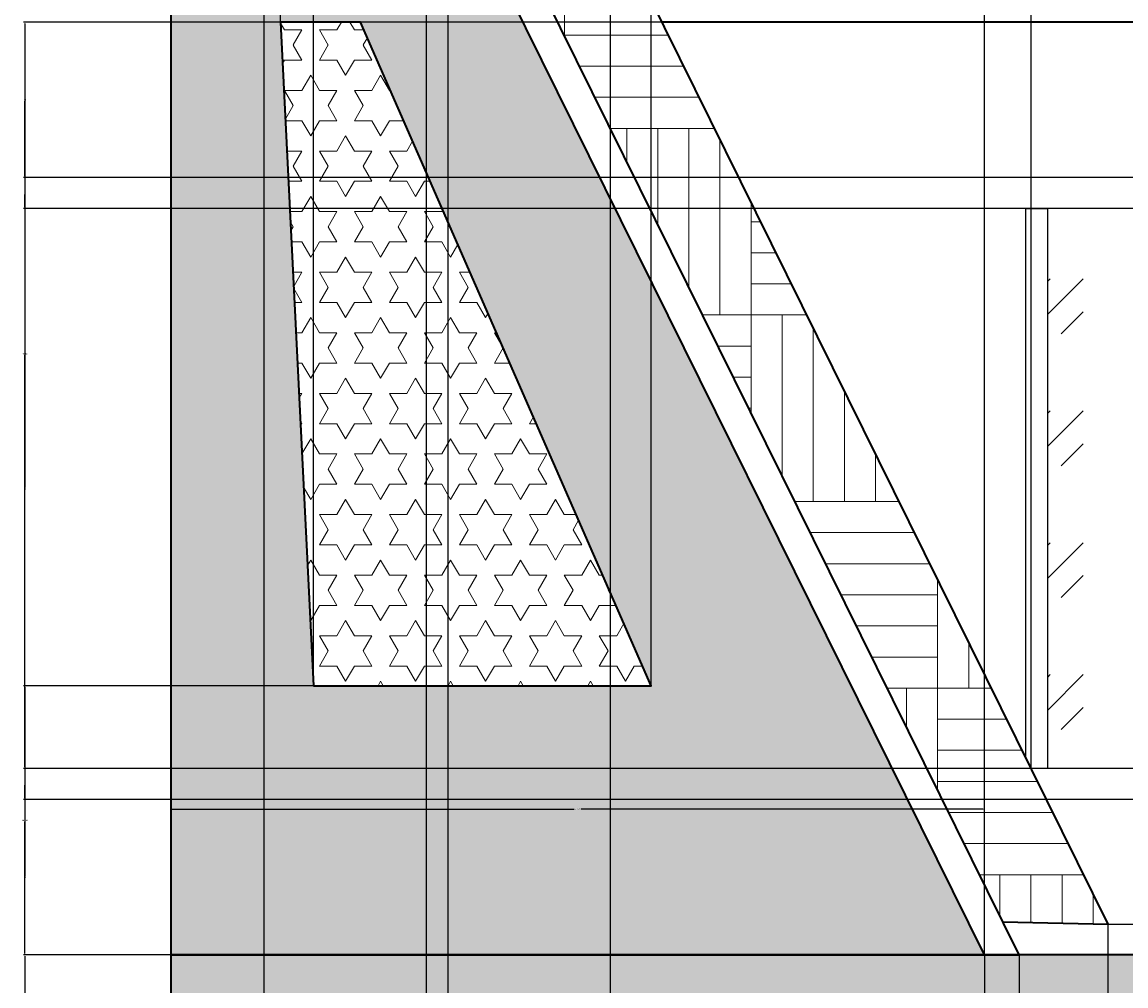
# Model space of a CAD drawing. Units: inches. Extents: x -9 to 389, y -55 to 344.
# Tile 2 of 5: x -9 to 133, y 119 to 243. Entities that reach past the tile are written whole.
import ezdxf

# ---------------------------------------------------------------- set-up
doc = ezdxf.new("R2010")
doc.units = ezdxf.units.IN
doc.header["$MEASUREMENT"] = 0
for name, color, linetype, lineweight in [('A-ANNO-DIMS', 2, 'Continuous', 18), ('A-ELEV', 7, 'Continuous', 35), ('A-ELEV-PATT', 8, 'Continuous', 13), ('A-GLAZ', 4, 'Continuous', 25), ('A-GLAZ-PATT', 252, 'Continuous', 13), ('A-ROOF', 1, 'Continuous', 35), ('A-ROOF-PATT', 8, 'Continuous', 13)]:
    doc.layers.add(name, color=color, linetype=linetype, lineweight=lineweight)
doc.styles.get("Standard").update_dxf_attribs({"font": 'arial.ttf'})
doc.dimstyles.get("Standard").update_dxf_attribs({"dimtxt": 0.18, "dimasz": 0.18, "dimexe": 0.18, "dimexo": 0.0625, "dimgap": 0.09, "dimtad": 0, "dimtih": 1, "dimtoh": 1, "dimdec": 4, "dimzin": 0, "dimdsep": 46, "dimtxsty": 'Standard', "dimcen": 0.09, "dimadec": 0, "dimazin": 0, "dimtfac": 1, "dimtdec": 4, "dimtofl": 0, "dimtmove": 0, "dimatfit": 3, "dimfxl": 1, "dimtolj": 1, "dimtzin": 0, "dimarcsym": 0})

# ---------------------------------------------------------------- blocks, each defined once
blk = doc.blocks.new('*D2')
at = {"layer": 'A-ANNO-DIMS', "color": 0, "lineweight": -2, "transparency": 16777216}
for p, q in [((23.77, 242.83), (23.77, 343.8)), ((23.95, 343.62), (25.5, 343.62)), ((27.83, 343.62), (26.29, 343.62)), ((28.01, 157.47), (28.01, 343.8))]:
    blk.add_line(p, q, dxfattribs=at)
at = {"layer": 'A-ANNO-DIMS', "color": 0, "transparency": 16777216}
for points in [[(23.95, 343.65), (23.95, 343.59), (23.77, 343.62)], [(27.83, 343.65), (27.83, 343.59), (28.01, 343.62)]]:
    blk.add_solid(points, dxfattribs=at)
at = {"layer": 'Defpoints', "color": 0, "transparency": 16777216}
for p in [(28.01, 343.62), (23.77, 242.77), (28.01, 157.4)]:
    blk.add_point(p, dxfattribs=at)
at = {"layer": 'A-ANNO-DIMS', "color": 0, "transparency": 16777216, "insert": (25.89, 343.62), "char_height": 0.18, "attachment_point": 5}
blk.add_mtext('\\A1;4.244', dxfattribs=at)
blk = doc.blocks.new('*D3')
at = {"layer": 'A-ANNO-DIMS', "color": 0, "lineweight": -2, "transparency": 16777216}
for p, q in [((28.01, 157.47), (28.01, 343.8)), ((28.19, 343.62), (49.26, 343.62)), ((71.27, 343.62), (50.2, 343.62)), ((71.45, 157.47), (71.45, 343.8))]:
    blk.add_line(p, q, dxfattribs=at)
at = {"layer": 'A-ANNO-DIMS', "color": 0, "transparency": 16777216}
for points in [[(28.19, 343.65), (28.19, 343.59), (28.01, 343.62)], [(71.27, 343.65), (71.27, 343.59), (71.45, 343.62)]]:
    blk.add_solid(points, dxfattribs=at)
at = {"layer": 'Defpoints', "color": 0, "transparency": 16777216}
for p in [(71.45, 343.62), (28.01, 157.4), (71.45, 157.4)]:
    blk.add_point(p, dxfattribs=at)
at = {"layer": 'A-ANNO-DIMS', "color": 0, "transparency": 16777216, "insert": (49.73, 343.62), "char_height": 0.18, "attachment_point": 5}
blk.add_mtext('\\A1;43.435', dxfattribs=at)
blk = doc.blocks.new('*D4')
at = {"layer": 'A-ANNO-DIMS', "color": 0, "lineweight": -2, "transparency": 16777216}
for p, q in [((71.45, 157.47), (71.45, 343.8)), ((71.63, 343.62), (119.03, 343.62)), ((167.08, 343.62), (119.68, 343.62)), ((167.26, 324.93), (167.26, 343.8))]:
    blk.add_line(p, q, dxfattribs=at)
at = {"layer": 'A-ANNO-DIMS', "color": 0, "transparency": 16777216}
for points in [[(71.63, 343.65), (71.63, 343.59), (71.45, 343.62)], [(167.08, 343.65), (167.08, 343.59), (167.26, 343.62)]]:
    blk.add_solid(points, dxfattribs=at)
at = {"layer": 'Defpoints', "color": 0, "transparency": 16777216}
for p in [(167.26, 343.62), (167.26, 324.87), (71.45, 157.4)]:
    blk.add_point(p, dxfattribs=at)
at = {"layer": 'A-ANNO-DIMS', "color": 0, "transparency": 16777216, "insert": (119.35, 343.62), "char_height": 0.18, "attachment_point": 5}
blk.add_mtext('\\A1;95.8', dxfattribs=at)
blk = doc.blocks.new('*D16')
at = {"layer": 'A-ANNO-DIMS', "color": 0, "lineweight": -2, "transparency": 16777216}
for p, q in [((21.65, 14.83), (21.65, 343.8)), ((21.83, 343.62), (31.64, 343.62)), ((42.37, 343.62), (32.57, 343.62)), ((42.55, 14.83), (42.55, 343.8))]:
    blk.add_line(p, q, dxfattribs=at)
at = {"layer": 'A-ANNO-DIMS', "color": 0, "transparency": 16777216}
for points in [[(21.83, 343.65), (21.83, 343.59), (21.65, 343.62)], [(42.37, 343.65), (42.37, 343.59), (42.55, 343.62)]]:
    blk.add_solid(points, dxfattribs=at)
at = {"layer": 'Defpoints', "color": 0, "transparency": 16777216}
for p in [(42.55, 343.62), (21.65, 14.77), (42.55, 14.77)]:
    blk.add_point(p, dxfattribs=at)
at = {"layer": 'A-ANNO-DIMS', "color": 0, "transparency": 16777216, "insert": (32.1, 343.62), "char_height": 0.18, "attachment_point": 5}
blk.add_mtext('\\A1;20.896', dxfattribs=at)
blk = doc.blocks.new('*D17')
at = {"layer": 'A-ANNO-DIMS', "color": 0, "lineweight": -2, "transparency": 16777216}
for p, q in [((42.55, 14.83), (42.55, 343.8)), ((42.73, 343.62), (43.61, 343.62)), ((45.14, 343.62), (44.26, 343.62)), ((45.32, 14.83), (45.32, 343.8))]:
    blk.add_line(p, q, dxfattribs=at)
at = {"layer": 'A-ANNO-DIMS', "color": 0, "transparency": 16777216}
for points in [[(42.73, 343.65), (42.73, 343.59), (42.55, 343.62)], [(45.14, 343.65), (45.14, 343.59), (45.32, 343.62)]]:
    blk.add_solid(points, dxfattribs=at)
at = {"layer": 'Defpoints', "color": 0, "transparency": 16777216}
for p in [(45.32, 343.62), (42.55, 14.77), (45.32, 14.77)]:
    blk.add_point(p, dxfattribs=at)
at = {"layer": 'A-ANNO-DIMS', "color": 0, "transparency": 16777216, "insert": (43.93, 343.62), "char_height": 0.18, "attachment_point": 5}
blk.add_mtext('\\A1;2.77', dxfattribs=at)
blk = doc.blocks.new('*D18')
at = {"layer": 'A-ANNO-DIMS', "color": 0, "lineweight": -2, "transparency": 16777216}
for p, q in [((45.32, 14.83), (45.32, 343.8)), ((45.5, 343.62), (55.3, 343.62)), ((66.03, 343.62), (56.23, 343.62)), ((66.21, 14.83), (66.21, 343.8))]:
    blk.add_line(p, q, dxfattribs=at)
at = {"layer": 'A-ANNO-DIMS', "color": 0, "transparency": 16777216}
for points in [[(45.5, 343.65), (45.5, 343.59), (45.32, 343.62)], [(66.03, 343.65), (66.03, 343.59), (66.21, 343.62)]]:
    blk.add_solid(points, dxfattribs=at)
at = {"layer": 'Defpoints', "color": 0, "transparency": 16777216}
for p in [(66.21, 343.62), (45.32, 14.77), (66.21, 14.77)]:
    blk.add_point(p, dxfattribs=at)
at = {"layer": 'A-ANNO-DIMS', "color": 0, "transparency": 16777216, "insert": (55.77, 343.62), "char_height": 0.18, "attachment_point": 5}
blk.add_mtext('\\A1;20.896', dxfattribs=at)
blk = doc.blocks.new('*D19')
at = {"layer": 'A-ANNO-DIMS', "color": 0, "lineweight": -2, "transparency": 16777216}
for p, q in [((66.21, 14.83), (66.21, 343.8)), ((66.39, 343.62), (109.71, 343.62)), ((153.81, 343.62), (110.5, 343.62)), ((153.99, 14.83), (153.99, 343.8))]:
    blk.add_line(p, q, dxfattribs=at)
at = {"layer": 'A-ANNO-DIMS', "color": 0, "transparency": 16777216}
for points in [[(66.39, 343.65), (66.39, 343.59), (66.21, 343.62)], [(153.81, 343.65), (153.81, 343.59), (153.99, 343.62)]]:
    blk.add_solid(points, dxfattribs=at)
at = {"layer": 'Defpoints', "color": 0, "transparency": 16777216}
for p in [(153.99, 343.62), (66.21, 14.77), (153.99, 14.77)]:
    blk.add_point(p, dxfattribs=at)
at = {"layer": 'A-ANNO-DIMS', "color": 0, "transparency": 16777216, "insert": (110.1, 343.62), "char_height": 0.18, "attachment_point": 5}
blk.add_mtext('\\A1;87.77', dxfattribs=at)
blk = doc.blocks.new('*D23')
at = {"layer": 'A-ANNO-DIMS', "color": 0, "lineweight": -2, "transparency": 16777216}
for p, q in [((9.59, 122.77), (-9.28, 122.77)), ((-9.1, 122.59), (-9.1, 116.95)), ((-9.1, 110.95), (-9.1, 116.59)), ((21.59, 110.77), (-9.28, 110.77))]:
    blk.add_line(p, q, dxfattribs=at)
at = {"layer": 'A-ANNO-DIMS', "color": 0, "transparency": 16777216}
for points in [[(-9.13, 122.59), (-9.07, 122.59), (-9.1, 122.77)], [(-9.13, 110.95), (-9.07, 110.95), (-9.1, 110.77)]]:
    blk.add_solid(points, dxfattribs=at)
at = {"layer": 'Defpoints', "color": 0, "transparency": 16777216}
for p in [(-9.1, 122.77), (9.65, 122.77), (21.65, 110.77)]:
    blk.add_point(p, dxfattribs=at)
at = {"layer": 'A-ANNO-DIMS', "color": 0, "transparency": 16777216, "insert": (-9.1, 116.77), "char_height": 0.18, "attachment_point": 5}
blk.add_mtext('\\A1;12', dxfattribs=at)
blk = doc.blocks.new('*D24')
at = {"layer": 'A-ANNO-DIMS', "color": 0, "lineweight": -2, "transparency": 16777216}
for p, q in [((27.95, 157.4), (-9.28, 157.4)), ((-9.1, 157.22), (-9.1, 140.27)), ((-9.1, 122.95), (-9.1, 139.9)), ((9.59, 122.77), (-9.28, 122.77))]:
    blk.add_line(p, q, dxfattribs=at)
at = {"layer": 'A-ANNO-DIMS', "color": 0, "transparency": 16777216}
for points in [[(-9.13, 157.22), (-9.07, 157.22), (-9.1, 157.4)], [(-9.13, 122.95), (-9.07, 122.95), (-9.1, 122.77)]]:
    blk.add_solid(points, dxfattribs=at)
at = {"layer": 'Defpoints', "color": 0, "transparency": 16777216}
for p in [(-9.1, 157.4), (28.01, 157.4), (9.65, 122.77)]:
    blk.add_point(p, dxfattribs=at)
at = {"layer": 'A-ANNO-DIMS', "color": 0, "transparency": 16777216, "insert": (-9.1, 140.09), "char_height": 0.18, "attachment_point": 5}
blk.add_mtext('\\A1;34.636', dxfattribs=at)
blk = doc.blocks.new('*D25')
at = {"layer": 'A-ANNO-DIMS', "color": 0, "lineweight": -2, "transparency": 16777216}
for p, q in [((23.71, 242.77), (-9.28, 242.77)), ((-9.1, 242.59), (-9.1, 200.27)), ((-9.1, 157.58), (-9.1, 199.9)), ((27.95, 157.4), (-9.28, 157.4))]:
    blk.add_line(p, q, dxfattribs=at)
at = {"layer": 'A-ANNO-DIMS', "color": 0, "transparency": 16777216}
for points in [[(-9.13, 242.59), (-9.07, 242.59), (-9.1, 242.77)], [(-9.13, 157.58), (-9.07, 157.58), (-9.1, 157.4)]]:
    blk.add_solid(points, dxfattribs=at)
at = {"layer": 'Defpoints', "color": 0, "transparency": 16777216}
for p in [(-9.1, 242.77), (23.77, 242.77), (28.01, 157.4)]:
    blk.add_point(p, dxfattribs=at)
at = {"layer": 'A-ANNO-DIMS', "color": 0, "transparency": 16777216, "insert": (-9.1, 200.09), "char_height": 0.18, "attachment_point": 5}
blk.add_mtext('\\A1;85.36', dxfattribs=at)
blk = doc.blocks.new('*D32')
at = {"layer": 'A-ANNO-DIMS', "color": 0, "lineweight": -2, "transparency": 16777216}
for p, q in [((9.65, 122.83), (9.65, 141.7)), ((9.83, 141.52), (61.53, 141.52)), ((114.14, 141.52), (62.44, 141.52)), ((114.32, 122.83), (114.32, 141.7))]:
    blk.add_line(p, q, dxfattribs=at)
at = {"layer": 'A-ANNO-DIMS', "color": 0, "transparency": 16777216}
for points in [[(9.83, 141.55), (9.83, 141.49), (9.65, 141.52)], [(114.14, 141.55), (114.14, 141.49), (114.32, 141.52)]]:
    blk.add_solid(points, dxfattribs=at)
at = {"layer": 'Defpoints', "color": 0, "transparency": 16777216}
for p in [(114.32, 141.52), (9.65, 122.77), (114.32, 122.77)]:
    blk.add_point(p, dxfattribs=at)
at = {"layer": 'A-ANNO-DIMS', "color": 0, "transparency": 16777216, "insert": (61.99, 141.52), "char_height": 0.18, "attachment_point": 5}
blk.add_mtext('\\A1;104.67', dxfattribs=at)
blk = doc.blocks.new('*D45')
at = {"layer": 'A-ANNO-DIMS', "color": 0, "lineweight": -2, "transparency": 16777216}
for p, q in [((122.22, 142.77), (-9.28, 142.77)), ((-9.1, 142.59), (-9.1, 132.95)), ((-9.1, 122.95), (-9.1, 132.59)), ((114.26, 122.77), (-9.28, 122.77))]:
    blk.add_line(p, q, dxfattribs=at)
at = {"layer": 'A-ANNO-DIMS', "color": 0, "transparency": 16777216}
for points in [[(-9.13, 142.59), (-9.07, 142.59), (-9.1, 142.77)], [(-9.13, 122.95), (-9.07, 122.95), (-9.1, 122.77)]]:
    blk.add_solid(points, dxfattribs=at)
at = {"layer": 'Defpoints', "color": 0, "transparency": 16777216}
for p in [(-9.1, 142.77), (122.28, 142.77), (114.32, 122.77)]:
    blk.add_point(p, dxfattribs=at)
at = {"layer": 'A-ANNO-DIMS', "color": 0, "transparency": 16777216, "insert": (-9.1, 132.77), "char_height": 0.18, "attachment_point": 5}
blk.add_mtext('\\A1;20', dxfattribs=at)
blk = doc.blocks.new('*D46')
at = {"layer": 'A-ANNO-DIMS', "color": 0, "lineweight": -2, "transparency": 16777216}
for p, q in [((120.238568, 146.768105), (-9.276734, 146.768105)), ((-9.096734, 146.588105), (-9.096734, 144.948105)), ((-9.096734, 142.948105), (-9.096734, 144.588105)), ((122.216644, 142.768105), (-9.276734, 142.768105))]:
    blk.add_line(p, q, dxfattribs=at)
at = {"layer": 'A-ANNO-DIMS', "color": 0, "transparency": 16777216}
for points in [[(-9.126734, 146.588105), (-9.066734, 146.588105), (-9.096734, 146.768105)], [(-9.126734, 142.948105), (-9.066734, 142.948105), (-9.096734, 142.768105)]]:
    blk.add_solid(points, dxfattribs=at)
at = {"layer": 'Defpoints', "color": 0, "transparency": 16777216}
for p in [(-9.096734, 146.768105), (120.301068, 146.768105), (122.279144, 142.768105)]:
    blk.add_point(p, dxfattribs=at)
at = {"layer": 'A-ANNO-DIMS', "color": 0, "transparency": 16777216, "insert": (-9.096734, 144.768105), "char_height": 0.18, "attachment_point": 5}
blk.add_mtext('\\A1;4', dxfattribs=at)
blk = doc.blocks.new('*D47')
at = {"layer": 'A-ANNO-DIMS', "color": 0, "lineweight": -2, "transparency": 16777216}
for p, q in [((84.63, 218.77), (-9.28, 218.77)), ((-9.1, 218.59), (-9.1, 182.95)), ((-9.1, 146.95), (-9.1, 182.59)), ((120.24, 146.77), (-9.28, 146.77))]:
    blk.add_line(p, q, dxfattribs=at)
at = {"layer": 'A-ANNO-DIMS', "color": 0, "transparency": 16777216}
for points in [[(-9.13, 218.59), (-9.07, 218.59), (-9.1, 218.77)], [(-9.13, 146.95), (-9.07, 146.95), (-9.1, 146.77)]]:
    blk.add_solid(points, dxfattribs=at)
at = {"layer": 'Defpoints', "color": 0, "transparency": 16777216}
for p in [(-9.1, 218.77), (84.7, 218.77), (120.3, 146.77)]:
    blk.add_point(p, dxfattribs=at)
at = {"layer": 'A-ANNO-DIMS', "color": 0, "transparency": 16777216, "insert": (-9.1, 182.77), "char_height": 0.18, "attachment_point": 5}
blk.add_mtext('\\A1;72', dxfattribs=at)
blk = doc.blocks.new('*D48')
at = {"layer": 'A-ANNO-DIMS', "color": 0, "lineweight": -2, "transparency": 16777216}
for p, q in [((82.655126, 222.768105), (-9.276734, 222.768105)), ((-9.096734, 222.588105), (-9.096734, 220.948105)), ((-9.096734, 218.948105), (-9.096734, 220.588105)), ((84.633202, 218.768105), (-9.276734, 218.768105))]:
    blk.add_line(p, q, dxfattribs=at)
at = {"layer": 'A-ANNO-DIMS', "color": 0, "transparency": 16777216}
for points in [[(-9.126734, 222.588105), (-9.066734, 222.588105), (-9.096734, 222.768105)], [(-9.126734, 218.948105), (-9.066734, 218.948105), (-9.096734, 218.768105)]]:
    blk.add_solid(points, dxfattribs=at)
at = {"layer": 'Defpoints', "color": 0, "transparency": 16777216}
for p in [(-9.096734, 222.768105), (82.717626, 222.768105), (84.695702, 218.768105)]:
    blk.add_point(p, dxfattribs=at)
at = {"layer": 'A-ANNO-DIMS', "color": 0, "transparency": 16777216, "insert": (-9.096734, 220.768105), "char_height": 0.18, "attachment_point": 5}
blk.add_mtext('\\A1;4', dxfattribs=at)
blk = doc.blocks.new('*D49')
at = {"layer": 'A-ANNO-DIMS', "color": 0, "lineweight": -2, "transparency": 16777216}
for p, q in [((72.76, 242.77), (-9.28, 242.77)), ((-9.1, 242.59), (-9.1, 232.95)), ((-9.1, 222.95), (-9.1, 232.59)), ((82.66, 222.77), (-9.28, 222.77))]:
    blk.add_line(p, q, dxfattribs=at)
at = {"layer": 'A-ANNO-DIMS', "color": 0, "transparency": 16777216}
for points in [[(-9.13, 242.59), (-9.07, 242.59), (-9.1, 242.77)], [(-9.13, 222.95), (-9.07, 222.95), (-9.1, 222.77)]]:
    blk.add_solid(points, dxfattribs=at)
at = {"layer": 'Defpoints', "color": 0, "transparency": 16777216}
for p in [(-9.1, 242.77), (72.83, 242.77), (82.72, 222.77)]:
    blk.add_point(p, dxfattribs=at)
at = {"layer": 'A-ANNO-DIMS', "color": 0, "transparency": 16777216, "insert": (-9.1, 232.77), "char_height": 0.18, "attachment_point": 5}
blk.add_mtext('\\A1;20', dxfattribs=at)
blk = doc.blocks.new('*D57')
at = {"layer": 'A-ANNO-DIMS', "color": 0, "lineweight": -2, "transparency": 16777216}
for p, q in [((114.32, 122.83), (114.32, 343.8)), ((114.5, 343.62), (116.93, 343.62)), ((120.12, 343.62), (117.69, 343.62)), ((120.3, 146.83), (120.3, 343.8))]:
    blk.add_line(p, q, dxfattribs=at)
at = {"layer": 'A-ANNO-DIMS', "color": 0, "transparency": 16777216}
for points in [[(114.5, 343.65), (114.5, 343.59), (114.32, 343.62)], [(120.12, 343.65), (120.12, 343.59), (120.3, 343.62)]]:
    blk.add_solid(points, dxfattribs=at)
at = {"layer": 'Defpoints', "color": 0, "transparency": 16777216}
for p in [(120.3, 343.62), (120.3, 146.77), (114.32, 122.77)]:
    blk.add_point(p, dxfattribs=at)
at = {"layer": 'A-ANNO-DIMS', "color": 0, "transparency": 16777216, "insert": (117.31, 343.62), "char_height": 0.18, "attachment_point": 5}
blk.add_mtext('\\A1;5.981', dxfattribs=at)
blk = doc.blocks.new('*D58')
at = {"layer": 'A-ANNO-DIMS', "color": 0, "lineweight": -2, "transparency": 16777216}
for p, q in [((120.3, 146.83), (120.3, 343.8)), ((120.48, 343.62), (131.33, 343.62)), ((143.12, 343.62), (132.26, 343.62)), ((143.3, 146.83), (143.3, 343.8))]:
    blk.add_line(p, q, dxfattribs=at)
at = {"layer": 'A-ANNO-DIMS', "color": 0, "transparency": 16777216}
for points in [[(120.48, 343.65), (120.48, 343.59), (120.3, 343.62)], [(143.12, 343.65), (143.12, 343.59), (143.3, 343.62)]]:
    blk.add_solid(points, dxfattribs=at)
at = {"layer": 'Defpoints', "color": 0, "transparency": 16777216}
for p in [(143.3, 343.62), (120.3, 146.77), (143.3, 146.77)]:
    blk.add_point(p, dxfattribs=at)
at = {"layer": 'A-ANNO-DIMS', "color": 0, "transparency": 16777216, "insert": (131.8, 343.62), "char_height": 0.18, "attachment_point": 5}
blk.add_mtext('\\A1;22.994', dxfattribs=at)
blk = doc.blocks.new('*D64')
at = {"layer": 'A-ANNO-DIMS', "color": 0, "lineweight": -2, "transparency": 16777216}
for p, q in [((130.27, 126.74), (388.58, 126.74)), ((388.4, 126.56), (388.4, 124.94)), ((388.4, 122.95), (388.4, 124.57)), ((118.84, 122.77), (388.58, 122.77))]:
    blk.add_line(p, q, dxfattribs=at)
at = {"layer": 'A-ANNO-DIMS', "color": 0, "transparency": 16777216}
for points in [[(388.37, 126.56), (388.43, 126.56), (388.4, 126.74)], [(388.37, 122.95), (388.43, 122.95), (388.4, 122.77)]]:
    blk.add_solid(points, dxfattribs=at)
at = {"layer": 'Defpoints', "color": 0, "transparency": 16777216}
for p in [(130.2, 126.74), (388.4, 126.74), (118.78, 122.77)]:
    blk.add_point(p, dxfattribs=at)
at = {"layer": 'A-ANNO-DIMS', "color": 0, "transparency": 16777216, "insert": (388.4, 124.76), "char_height": 0.18, "attachment_point": 5}
blk.add_mtext('\\A1;3.976', dxfattribs=at)
blk = doc.blocks.new('*D65')
at = {"layer": 'A-ANNO-DIMS', "color": 0, "lineweight": -2, "transparency": 16777216}
for p, q in [((130.2, 126.68), (130.2, -54.92)), ((118.78, 122.71), (118.78, -54.92)), ((118.96, -54.74), (124.11, -54.74)), ((130.02, -54.74), (124.88, -54.74))]:
    blk.add_line(p, q, dxfattribs=at)
at = {"layer": 'A-ANNO-DIMS', "color": 0, "transparency": 16777216}
for points in [[(118.96, -54.71), (118.96, -54.77), (118.78, -54.74)], [(130.02, -54.71), (130.02, -54.77), (130.2, -54.74)]]:
    blk.add_solid(points, dxfattribs=at)
at = {"layer": 'Defpoints', "color": 0, "transparency": 16777216}
for p in [(130.2, 126.74), (118.78, 122.77), (130.2, -54.74)]:
    blk.add_point(p, dxfattribs=at)
at = {"layer": 'A-ANNO-DIMS', "color": 0, "transparency": 16777216, "insert": (124.49, -54.74), "char_height": 0.18, "attachment_point": 5}
blk.add_mtext('\\A1;11.42', dxfattribs=at)
blk = doc.blocks.new('*D68')
at = {"layer": 'A-ANNO-DIMS', "color": 0, "lineweight": -2, "transparency": 16777216}
for p, q in [((114.32, 122.71), (114.32, -54.92)), ((289.4, 122.71), (289.4, -54.92)), ((114.5, -54.74), (201.4, -54.74)), ((289.22, -54.74), (202.31, -54.74))]:
    blk.add_line(p, q, dxfattribs=at)
at = {"layer": 'A-ANNO-DIMS', "color": 0, "transparency": 16777216}
for points in [[(114.5, -54.71), (114.5, -54.77), (114.32, -54.74)], [(289.22, -54.71), (289.22, -54.77), (289.4, -54.74)]]:
    blk.add_solid(points, dxfattribs=at)
at = {"layer": 'Defpoints', "color": 0, "transparency": 16777216}
for p in [(114.32, 122.77), (289.4, 122.77), (289.4, -54.74)]:
    blk.add_point(p, dxfattribs=at)
at = {"layer": 'A-ANNO-DIMS', "color": 0, "transparency": 16777216, "insert": (201.86, -54.74), "char_height": 0.18, "attachment_point": 5}
blk.add_mtext('\\A1;175.08', dxfattribs=at)

msp = doc.modelspace()

# ---------------------------------------------------------------- hatches: boundary and pattern name
at = {"layer": 'A-ELEV-PATT'}
h = msp.add_hatch(color=256, dxfattribs=at)
h.dxf.hatch_style = 1
h.paths.add_polyline_path([(35.4778, 282.2003), (9.6533, 282.2003), (9.6533, 122.7681), (114.32, 122.7681)])
h.paths.add_polyline_path([(28.0148, 157.4044), (23.771, 242.7681), (34.0623, 242.7681), (71.4494, 157.4044)], flags=16)
h = msp.add_hatch(dxfattribs=at)
h.set_pattern_fill('STARS', color=256, scale=18)
h.set_pattern_definition([(0, (-83.729, -34.93), (0, 3.897114), [2.25, -2.25]), (60, (-83.729, -34.93), (-3.375, 1.948557), [2.25, -2.25]), (120, (-82.604, -32.9816), (-3.375, -1.948557), [2.25, -2.25])])
h.paths.add_polyline_path([(34.0623, 242.7681), (23.771, 242.7681), (28.0148, 157.4044), (71.4494, 157.4044)])
h = msp.add_hatch(color=256, dxfattribs=at)
h.dxf.hatch_style = 1
h.paths.add_polyline_path([(369.6533, 122.7681), (289.3963, 122.7681), (9.6533, 122.7681), (9.6533, 2.7681), (369.6533, 2.7681)])
h.paths.add_polyline_path([(177.6533, 110.7681), (177.6533, 14.7681), (21.6533, 14.7681), (21.6533, 110.7681)], flags=16)
h.paths.add_polyline_path([(201.6533, 110.7681), (357.6533, 110.7681), (357.6533, 14.7681), (201.6533, 14.7681)], flags=16)
h.paths.add_polyline_path([(156.7573, 110.7681), (156.7573, 14.7681), (153.9877, 14.7681), (153.9877, 110.7681)], flags=0)
h.paths.add_polyline_path([(222.5492, 110.7681), (225.3188, 110.7681), (225.3188, 14.7681), (222.5492, 14.7681)], flags=0)
h.paths.add_polyline_path([(246.2148, 110.7681), (248.9844, 110.7681), (248.9844, 14.7681), (246.2148, 14.7681)], flags=0)
h.paths.add_polyline_path([(269.8803, 110.7681), (272.65, 110.7681), (272.65, 14.7681), (269.8803, 14.7681)], flags=0)
h.paths.add_polyline_path([(68.9844, 110.7681), (68.9844, 14.7681), (66.2148, 14.7681), (66.2148, 110.7681)], flags=0)
h.paths.add_polyline_path([(45.3188, 110.7681), (45.3188, 14.7681), (42.5492, 14.7681), (42.5492, 110.7681)], flags=0)
at = {"layer": 'A-GLAZ-PATT', "transparency": 33554536}
h = msp.add_hatch(dxfattribs=at)
h.set_pattern_fill('GOST_GLASS', color=256, scale=2)
h.set_pattern_definition([(45, (-83.729, -34.93), (16.97056, 0), [10, -14]), (45, (-79.486, -34.93), (16.97056, 0), [4, -20]), (45, (-83.729, -30.687), (16.97056, 0), [4, -20])])
h.paths.add_polyline_path([(153.9877, 110.7681), (68.9844, 110.7681), (68.9844, 14.7681), (153.9877, 14.7681)])
h.paths.add_polyline_path([(357.6533, 110.7681), (272.65, 110.7681), (272.65, 14.7681), (357.6533, 14.7681)])
h.paths.add_polyline_path([(190.6266, 218.7681), (169.7307, 218.7681), (169.7307, 146.7681), (190.6266, 146.7681)])
h.paths.add_polyline_path([(143.2954, 218.7681), (122.3995, 218.7681), (122.3995, 146.7681), (143.2954, 146.7681)])
h.paths.add_polyline_path([(237.9578, 184.6816), (217.3576, 218.7681), (217.0618, 218.7681), (217.0618, 146.7681), (237.9578, 146.7681)])
h.paths.add_polyline_path([(42.5492, 110.7681), (21.6533, 110.7681), (21.6533, 14.7681), (42.5492, 14.7681)])
h.paths.add_polyline_path([(246.2148, 110.7681), (225.3188, 110.7681), (225.3188, 14.7681), (246.2148, 14.7681)])
at = {"layer": 'A-ROOF-PATT'}
h = msp.add_hatch(dxfattribs=at)
h.set_pattern_fill('AR-PARQ1', color=256, scale=2)
h.set_pattern_definition([(90, (-83.73, -34.93), (-24, 24), [24, -24]), (90, (-79.73, -34.93), (-24, 24), [24, -24]), (90, (-75.73, -34.93), (-24, 24), [24, -24]), (90, (-71.73, -34.93), (-24, 24), [24, -24]), (90, (-67.73, -34.93), (-24, 24), [24, -24]), (90, (-63.73, -34.93), (-24, 24), [24, -24]), (90, (-59.73, -34.93), (-24, 24), [24, -24]), (0, (-83.73, -10.93), (24, -24), [24, -24]), (0, (-83.73, -6.93), (24, -24), [24, -24]), (0, (-83.73, -2.93), (24, -24), [24, -24]), (0, (-83.73, 1.07), (24, -24), [24, -24]), (0, (-83.73, 5.07), (24, -24), [24, -24]), (0, (-83.73, 9.07), (24, -24), [24, -24]), (0, (-83.73, 13.07), (24, -24), [24, -24])])
h.paths.add_polyline_path([(59.2615, 270.2003), (45.8744, 270.2003), (116.6802, 127.0192), (130.2035, 126.7437)])
h.paths.add_polyline_path([(174.5076, 312.8713), (160.4864, 312.8713), (271.5791, 129.0492), (285.7644, 128.7778)])

# ---------------------------------------------------------------- linework, layer by layer
at = {"layer": 'A-ELEV'}
for p, q in [((9.6533, 282.2003), (9.6533, 122.7681)), ((9.6533, 242.7681), (9.6533, 2.7681)), ((202.8532, 242.7681), (72.8272, 242.7681)), ((369.6533, 122.7681), (9.6533, 122.7681)), ((9.6533, 122.7681), (118.7824, 122.7681))]:
    msp.add_line(p, q, dxfattribs=at)
msp.add_lwpolyline([(28.0148, 157.4044), (71.4494, 157.4044), (34.0623, 242.7681), (23.771, 242.7681)], close=True, dxfattribs=at)
at = {"layer": 'A-GLAZ'}
for p, q in [((214.9402, 222.7681), (82.7176, 222.7681)), ((217.3576, 218.7681), (84.6957, 218.7681)), ((260.8707, 146.7681), (120.3011, 146.7681)), ((263.2881, 142.7681), (122.2791, 142.7681))]:
    msp.add_line(p, q, dxfattribs=at)
msp.add_lwpolyline([(119.6299, 148.1254), (119.6299, 218.7681), (122.3995, 218.7681), (122.3995, 146.7681)], dxfattribs=at)
at = {"layer": 'A-ROOF'}
for p, q in [((114.32, 122.7681), (35.4778, 282.2003)), ((118.7824, 122.7681), (39.9402, 282.2003)), ((130.2035, 126.7437), (59.2615, 270.2003)), ((116.6802, 127.0192), (130.2035, 126.7437))]:
    msp.add_line(p, q, dxfattribs=at)

# ---------------------------------------------------------------- dimensions: what is measured, and where the dimension line sits
at = {"layer": 'A-ANNO-DIMS'}
for base, p1, p2, override, picture, middle in [((42.5492, 343.6213), (21.6533, 14.7681), (42.5492, 14.7681), {"dimdec": 3, "dimlfac": 1, "dimrnd": 0, "dimzin": 0, "dimdsep": 46, "dimlunit": 2}, '*D16', (32.1012, 343.6213)), ((28.0148, 343.6213), (23.771, 242.7681), (28.0148, 157.4044), {"dimdec": 3, "dimlfac": 1, "dimrnd": 0, "dimzin": 0, "dimdsep": 46, "dimlunit": 2}, '*D2', (25.8929, 343.6213)), ((71.4494, 343.6213), (28.0148, 157.4044), (71.4494, 157.4044), {"dimdec": 3, "dimlfac": 1, "dimrnd": 0, "dimzin": 0, "dimdsep": 46, "dimlunit": 2}, '*D3', (49.7321, 343.6213)), ((45.3188, 343.6213), (42.5492, 14.7681), (45.3188, 14.7681), {"dimdec": 2, "dimlfac": 1, "dimrnd": 0, "dimzin": 0, "dimdsep": 46, "dimlunit": 2}, '*D17', (43.934, 343.6213)), ((66.2148, 343.6213), (45.3188, 14.7681), (66.2148, 14.7681), {"dimdec": 3, "dimlfac": 1, "dimrnd": 0, "dimzin": 0, "dimdsep": 46, "dimlunit": 2}, '*D18', (55.7668, 343.6213)), ((153.9877, 343.6213), (66.2148, 14.7681), (153.9877, 14.7681), {"dimdec": 2, "dimlfac": 1, "dimrnd": 0, "dimzin": 0, "dimdsep": 46, "dimlunit": 2}, '*D19', (110.1012, 343.6213)), ((167.2555, 343.6213), (71.4494, 157.4044), (167.2555, 324.8713), {"dimdec": 1, "dimlfac": 1, "dimrnd": 0, "dimzin": 0, "dimdsep": 46, "dimlunit": 2}, '*D4', (119.3525, 343.6213)), ((120.3011, 343.6213), (114.32, 122.7681), (120.3011, 146.7681), {"dimdec": 3, "dimlfac": 1, "dimrnd": 0, "dimzin": 0, "dimdsep": 46, "dimlunit": 2}, '*D57', (117.3105, 343.6213)), ((143.2954, 343.6213), (120.3011, 146.7681), (143.2954, 146.7681), {"dimdec": 3, "dimlfac": 1, "dimrnd": 0, "dimzin": 0, "dimdsep": 46, "dimlunit": 2}, '*D58', (131.7983, 343.6213)), ((114.32, 141.5181), (9.6533, 122.7681), (114.32, 122.7681), {"dimdec": 2, "dimlfac": 1, "dimrnd": 0, "dimzin": 0, "dimdsep": 46, "dimlunit": 2}, '*D32', (61.9866, 141.5181)), ((130.2035, -54.7386), (118.7824, 122.7681), (130.2035, 126.7437), {"dimdec": 2, "dimlfac": 1, "dimrnd": 0, "dimzin": 0, "dimdsep": 46, "dimlunit": 2}, '*D65', (124.493, -54.7386)), ((289.3963, -54.7386), (114.32, 122.7681), (289.3963, 122.7681), {"dimdec": 2, "dimlfac": 1, "dimrnd": 0, "dimzin": 0, "dimdsep": 46, "dimlunit": 2}, '*D68', (201.8582, -54.7386))]:
    dim = msp.add_linear_dim(base=base, p1=p1, p2=p2, dimstyle='Standard', override=override, dxfattribs=at)
    dim.commit()
    dim.dimension.update_dxf_attribs({"geometry": picture, "text_midpoint": middle})
for base, p1, p2, override, picture, middle in [((-9.0967, 242.7681), (28.0148, 157.4044), (23.771, 242.7681), {"dimdec": 2, "dimlfac": 1, "dimrnd": 0, "dimzin": 0, "dimdsep": 46, "dimlunit": 2}, '*D25', (-9.0967, 200.0863)), ((-9.0967, 242.7681), (82.7176, 222.7681), (72.8272, 242.7681), {"dimdec": 0, "dimlfac": 1, "dimrnd": 0, "dimzin": 0, "dimdsep": 46, "dimlunit": 2}, '*D49', (-9.0967, 232.7681)), ((-9.0967, 222.7681), (84.6957, 218.7681), (82.7176, 222.7681), {"dimdec": 0, "dimlfac": 1, "dimrnd": 0, "dimzin": 0, "dimdsep": 46, "dimlunit": 2}, '*D48', (-9.0967, 220.7681)), ((-9.0967, 218.7681), (120.3011, 146.7681), (84.6957, 218.7681), {"dimdec": 0, "dimlfac": 1, "dimrnd": 0, "dimzin": 0, "dimdsep": 46, "dimlunit": 2}, '*D47', (-9.0967, 182.7681)), ((-9.0967, 157.4044), (9.6533, 122.7681), (28.0148, 157.4044), {"dimdec": 3, "dimlfac": 1, "dimrnd": 0, "dimzin": 0, "dimdsep": 46, "dimlunit": 2}, '*D24', (-9.0967, 140.0863)), ((-9.0967, 146.7681), (122.2791, 142.7681), (120.3011, 146.7681), {"dimdec": 0, "dimlfac": 1, "dimrnd": 0, "dimzin": 0, "dimdsep": 46, "dimlunit": 2}, '*D46', (-9.0967, 144.7681)), ((-9.0967, 142.7681), (114.32, 122.7681), (122.2791, 142.7681), {"dimdec": 0, "dimlfac": 1, "dimrnd": 0, "dimzin": 0, "dimdsep": 46, "dimlunit": 2}, '*D45', (-9.0967, 132.7681)), ((388.4033, 126.7437), (118.7824, 122.7681), (130.2035, 126.7437), {"dimdec": 3, "dimlfac": 1, "dimrnd": 0, "dimzin": 0, "dimdsep": 46, "dimlunit": 2}, '*D64', (388.4033, 124.7559)), ((-9.0967, 122.7681), (21.6533, 110.7681), (9.6533, 122.7681), {"dimdec": 0, "dimlfac": 1, "dimrnd": 0, "dimzin": 0, "dimdsep": 46, "dimlunit": 2}, '*D23', (-9.0967, 116.7681))]:
    dim = msp.add_linear_dim(base=base, p1=p1, p2=p2, angle=90, dimstyle='Standard', override=override, dxfattribs=at)
    dim.commit()
    dim.dimension.update_dxf_attribs({"geometry": picture, "text_midpoint": middle})

doc.saveas('drawing.dxf')
